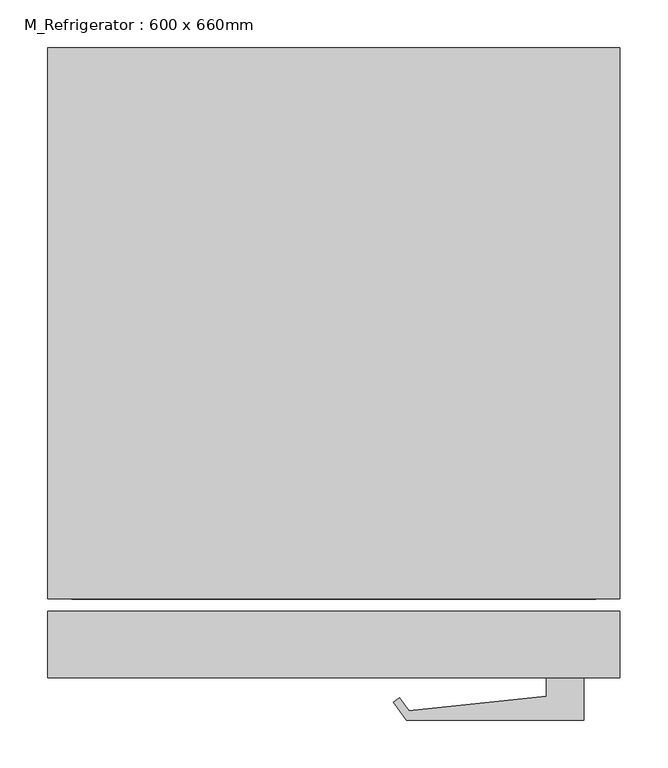
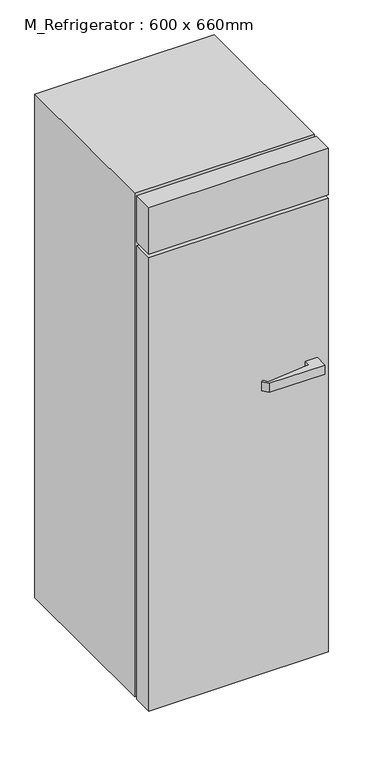
"""IFC4 building model written with IfcOpenShell, lengths in millimetres: proxy geometry, M_Refrigerator : 600 x 660mm."""

from ifc_helpers import new_model, si_unit, point, frame, frame_2d, origin, origin_with_axes, place, context, project, spatial, polyline, circle_curve, trimmed, segment, composite_curve, outline, extrude, source, transform, mapped, element, save


def m_refrigerator_600_x_660mm_a466bf94(model_context):
    return source(origin(), model_context, "Body", "SweptSolid", [
        extrude(outline(polyline([(208.0988574, -408.1036861), (22.3988574, -408.1036861), (8.7240737, -389.5368406), (15.2273026, -384.7471068), (25.1756383, -398.2543926), (168.9242419, -383.0358618), (168.9242419, -363.7849098), (208.0988574, -363.7849098), (208.0988574, -408.1036861)])), frame((0.0, 0.0, 1071.927792), z_axis=(0.0, 0.0, 1.0), x_axis=(1.0, 0.0, 0.0)), (0.0, 0.0, 1.0), 31.75),
        extrude(outline(composite_curve([segment(trimmed(circle_curve(frame_2d((-271.2511426, 220.0150902)), 25.4), [point((-296.6511426, 220.0150902))], [point((-245.8511426, 220.0150902))], False, "CARTESIAN"), True, "CONTINUOUS"), segment(trimmed(circle_curve(frame_2d((-271.2511426, 220.0150902)), 25.4), [point((-245.8511426, 220.0150902))], [point((-296.6511426, 220.0150902))], False, "CARTESIAN"), True, "CONTINUOUS")], self_intersect=False)), origin_with_axes(), (0.0, 0.0, 1.0), 50.8),
        extrude(outline(composite_curve([segment(trimmed(circle_curve(frame_2d((163.6488574, 220.0150902)), 25.4), [point((138.2488574, 220.0150902))], [point((189.0488574, 220.0150902))], False, "CARTESIAN"), True, "CONTINUOUS"), segment(trimmed(circle_curve(frame_2d((163.6488574, 220.0150902)), 25.4), [point((189.0488574, 220.0150902))], [point((138.2488574, 220.0150902))], False, "CARTESIAN"), True, "CONTINUOUS")], self_intersect=False)), origin_with_axes(), (0.0, 0.0, 1.0), 50.8),
        extrude(outline(composite_curve([segment(trimmed(circle_curve(frame_2d((-271.2511426, -236.7849098)), 25.4), [point((-296.6511426, -236.7849098))], [point((-245.8511426, -236.7849098))], False, "CARTESIAN"), True, "CONTINUOUS"), segment(trimmed(circle_curve(frame_2d((-271.2511426, -236.7849098)), 25.4), [point((-245.8511426, -236.7849098))], [point((-296.6511426, -236.7849098))], False, "CARTESIAN"), True, "CONTINUOUS")], self_intersect=False)), origin_with_axes(), (0.0, 0.0, 1.0), 50.8),
        extrude(outline(composite_curve([segment(trimmed(circle_curve(frame_2d((163.6488574, -236.7849098)), 25.4), [point((138.2488574, -236.7849098))], [point((189.0488574, -236.7849098))], False, "CARTESIAN"), True, "CONTINUOUS"), segment(trimmed(circle_curve(frame_2d((163.6488574, -236.7849098)), 25.4), [point((189.0488574, -236.7849098))], [point((138.2488574, -236.7849098))], False, "CARTESIAN"), True, "CONTINUOUS")], self_intersect=False)), origin_with_axes(), (0.0, 0.0, 1.0), 50.8),
        extrude(outline(polyline([(246.1988574, -363.7849098), (-353.8011426, -363.7849098), (-353.8011426, -293.9349098), (246.1988574, -293.9349098), (246.1988574, -363.7849098)])), frame((0.0, 0.0, 50.8), z_axis=(0.0, 0.0, 1.0), x_axis=(1.0, 0.0, 0.0)), (0.0, 0.0, 1.0), 1601.4),
        extrude(outline(polyline([(246.1988574, -363.7849098), (-353.8011426, -363.7849098), (-353.8011426, -293.9349098), (246.1988574, -293.9349098), (246.1988574, -363.7849098)])), frame((0.0, 0.0, 1664.9), z_axis=(0.0, 0.0, 1.0), x_axis=(1.0, 0.0, 0.0)), (0.0, 0.0, 1.0), 165.1),
        extrude(outline(polyline([(220.7988574, 270.8150902), (-328.4011426, 270.8150902), (-328.4011426, 296.2150902), (220.7988574, 296.2150902), (220.7988574, 270.8150902)])), frame((0.0, 0.0, 152.4), z_axis=(0.0, 0.0, 1.0), x_axis=(1.0, 0.0, 0.0)), (0.0, 0.0, 1.0), 1652.2),
        extrude(outline(polyline([(1830.0, 246.1988574), (1830.0, -353.8011426), (50.8, -353.8011426), (50.8, 246.1988574), (1830.0, 246.1988574)]), holes=[polyline([(1626.8, 220.7988574), (431.8, 220.7988574), (431.8, -328.4011426), (1626.8, -328.4011426), (1626.8, 220.7988574)])]), frame((0.0, -281.2349098, 0.0), z_axis=(0.0, 1.0, 0.0), x_axis=(0.0, 0.0, 1.0)), (0.0, 0.0, 1.0), 577.45),
    ])


if __name__ == "__main__":
    model = new_model("IFC4")
    model_context = context("Model", 3, world=origin())
    ifc_project = project(units=[si_unit("LENGTHUNIT", "METRE", prefix="MILLI")], contexts=[model_context])
    site = spatial("IfcSite", under=ifc_project)
    building = spatial("IfcBuilding", under=site)
    placement = place(None, origin())
    m_refrigerator_600_x_660mm_shape = m_refrigerator_600_x_660mm_a466bf94(model_context)
    element("IfcBuildingElementProxy", 1, Name="M_Refrigerator : 600 x 660mm", ObjectType="M_Refrigerator : 600 x 660mm", at=placement, inside=building, context=model_context, shape_type="MappedRepresentation", body=[
        mapped(m_refrigerator_600_x_660mm_shape, transform((0.0, 0.0, 0.0), x_axis=(1.0, 0.0, 0.0), y_axis=(0.0, 1.0, 0.0), z_axis=(0.0, 0.0, 1.0))),
    ])
    save(model, "model.ifc")

# Revit data of these elements
# Type "M_Refrigerator : 600 x 660mm"
#   Label = "REF."
#   Depth = 2' - 1.98425"
#   Height = 6' - 0.04724"
#   Width = 1' - 11.62205"
#   Material = Steel, Paint Finish, Ivory, Matte
#   Description = (empty or 0)
#   Default Elevation = 0
# Element 1 (IfcBuildingElementProxy, "M_Refrigerator : 600 x 660mm")
#   Materials on its faces: "Steel, Paint Finish, Ivory, Matte", "Steel, Chrome Plated"
# Materials
#   "Steel, Paint Finish, Ivory, Matte": class "Metal", colour RGB 247 247 239, transparency 0, Description = "Steel, paint finish, ivory, matte", Cost = 0
#   "Steel, Chrome Plated": class "Metal", colour RGB 17 17 17, transparency 0, Description = "Chromiuim plated steel", Cost = 0
